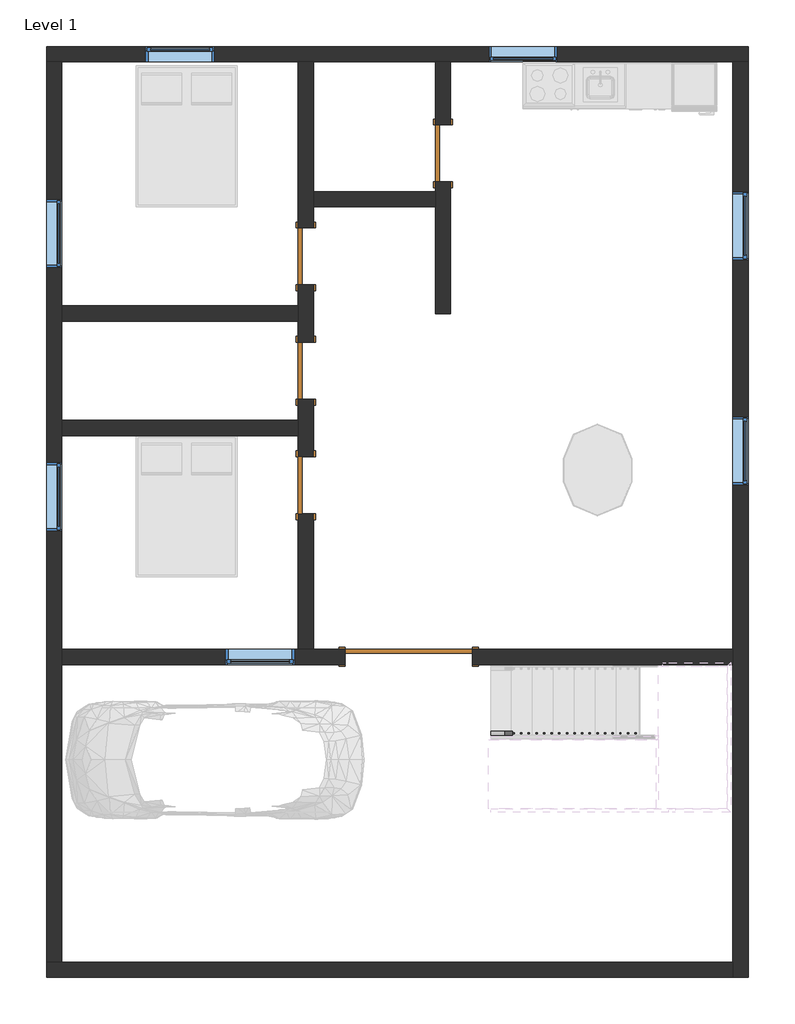
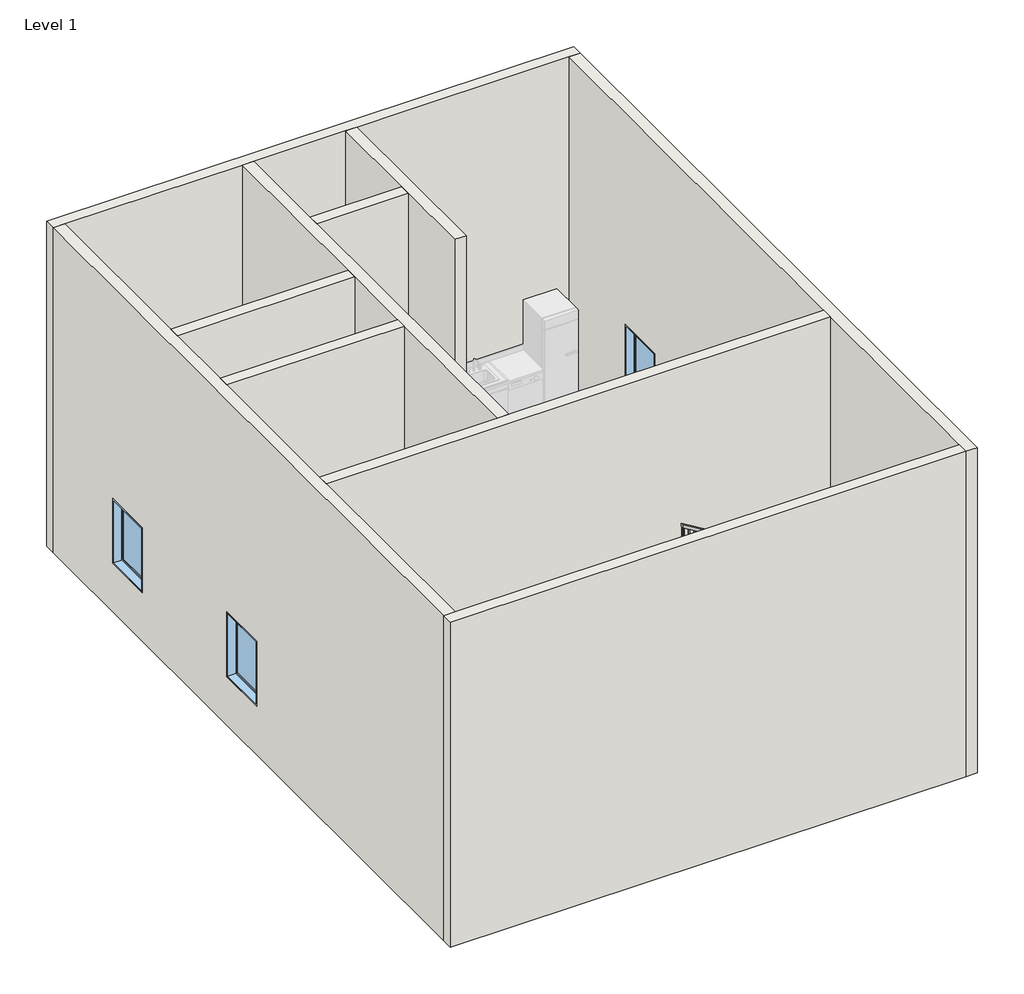
# One storey, part 1 of 2: 10 walls, 7 windows, 5 doors, 1 railing.
"""IFC4 building model written with IfcOpenShell, lengths in millimetres."""

from ifc_helpers import new_model, si_unit, frame, origin, origin_with_axes, place, context, project, spatial, polyline, outline, extrude, faceted_brep, transform, mapped, element, save
from components import m_door_double_flush_panel_double_acting_1700_x_2000mm_ee2ba557, door_53b1b562, door_fadea3f2, window_e2841890, window_9a779fa2

model = new_model("IFC4")

# Units and contexts
model_context = context("Model", 3, world=origin())
ifc_project = project(units=[si_unit("LENGTHUNIT", "METRE", prefix="MILLI")], contexts=[model_context])

# Site, building, storey
site = spatial("IfcSite", under=ifc_project)
building = spatial("IfcBuilding", under=site)
storey = spatial("IfcBuildingStorey", under=building, Name="Level 1", Elevation=0.0)

# Doors
placement = place(None, origin())
m_door_double_flush_panel_double_acting_1700_x_2000mm_shape = m_door_double_flush_panel_double_acting_1700_x_2000mm_ee2ba557(model_context)
element("IfcDoor", 1, ObjectType="M_Door-Double-Flush_Panel-Double-Acting : 1700 x 2000mm", at=placement, inside=storey, context=model_context, shape_type="MappedRepresentation", body=[
    mapped(m_door_double_flush_panel_double_acting_1700_x_2000mm_shape, transform((-5017.6851125, 2283.4979873, 0.0), x_axis=(1.0, 0.0, 0.0), y_axis=(0.0, 1.0, 0.0), z_axis=(0.0, 0.0, 1.0))),
])
door_shape = door_53b1b562(model_context)
element("IfcDoor", 2, ObjectType="Single-Flush : 30\" x 80\"", at=placement, inside=storey, context=model_context, shape_type="MappedRepresentation", body=[
    mapped(door_shape, transform((-4560.4851125, 8989.0979873, 0.0), x_axis=(0.0, -1.0, 0.0), y_axis=(1.0, 0.0, 0.0), z_axis=(0.0, 0.0, 1.0))),
])
element("IfcDoor", 3, ObjectType="Single-Flush : 30\" x 80\"", at=placement, inside=storey, context=model_context, shape_type="MappedRepresentation", body=[
    mapped(door_shape, transform((-6389.2851125, 7617.4979873, 0.0), x_axis=(0.0, -1.0, 0.0), y_axis=(1.0, 0.0, 0.0), z_axis=(0.0, 0.0, 1.0))),
])
door_2_shape = door_fadea3f2(model_context)
element("IfcDoor", 4, ObjectType="Single-Flush : 30\" x 80\"", at=placement, inside=storey, context=model_context, shape_type="MappedRepresentation", body=[
    mapped(door_2_shape, transform((-6389.2851125, 6093.4979873, 0.0), x_axis=(0.0, 1.0, 0.0), y_axis=(-1.0, 0.0, 0.0), z_axis=(0.0, 0.0, 1.0))),
])
element("IfcDoor", 5, ObjectType="Single-Flush : 30\" x 80\"", at=placement, inside=storey, context=model_context, shape_type="MappedRepresentation", body=[
    mapped(door_2_shape, transform((-6389.2851125, 4569.4979873, 0.0), x_axis=(0.0, 1.0, 0.0), y_axis=(-1.0, 0.0, 0.0), z_axis=(0.0, 0.0, 1.0))),
])

# Railing
element("IfcRailing", 6, ObjectType="Handrail - Rectangular", at=placement, inside=storey, context=model_context, shape_type="SolidModel", body=[
    faceted_brep([(-3925.4851125, 1292.9395264, 1083.7333333), (-3925.4851125, 1292.9395264, 1024.3318731), (-3925.4851125, 1242.1395264, 1024.3318731), (-3925.4851125, 1242.1395264, 1083.7333333), (-1766.4851125, 1292.9395264, 2392.2181818), (-1715.6851125, 1292.9395264, 2363.6046004), (-1715.6851125, 1242.1395264, 2363.6046004), (-1766.4851125, 1242.1395264, 2392.2181818), (-1766.4851125, 1292.9395264, 2438.4), (-1715.6851125, 1292.9395264, 2387.6), (-1715.6851125, 1242.1395264, 2387.6), (-1766.4851125, 1242.1395264, 2438.4), (-1639.4851125, 1292.9395264, 2438.4), (-1639.4851125, 1292.9395264, 2387.6), (-1690.2851125, 1242.1395264, 2387.6), (-1690.2851125, 1242.1395264, 2438.4), (-1639.4851125, 1165.9395264, 2438.4), (-1639.4851125, 1165.9395264, 2387.6), (-1690.2851125, 1165.9395264, 2387.6), (-1690.2851125, 1165.9395264, 2438.4), (-1639.4851125, 1153.7428815, 2438.4), (-1690.2851125, 1153.7428815, 2438.4), (-1690.2851125, 1153.7428815, 2387.6), (-1639.4851125, 1153.7428815, 2387.6)], [[[0, 1, 2, 3]], [[1, 0, 4, 5]], [[2, 1, 5, 6]], [[3, 2, 6, 7]], [[0, 3, 7, 4]], [[5, 4, 8, 9]], [[6, 5, 9, 10]], [[7, 6, 10, 11]], [[4, 7, 11, 8]], [[9, 8, 12, 13]], [[10, 9, 13, 14]], [[11, 10, 14, 15]], [[8, 11, 15, 12]], [[13, 12, 16, 17]], [[14, 13, 17, 18]], [[15, 14, 18, 19]], [[12, 15, 19, 16]], [[20, 21, 22, 23]], [[17, 16, 20, 23]], [[18, 17, 23, 22]], [[19, 18, 22, 21]], [[16, 19, 21, 20]]]),
    faceted_brep([(-1639.4851125, 1179.1428815, 2438.4), (-1639.4851125, 1128.3428815, 2387.6), (-1690.2851125, 1128.3428815, 2387.6), (-1690.2851125, 1179.1428815, 2438.4), (-1639.4851125, 1179.1428815, 2576.9454545), (-1690.2851125, 1179.1428815, 2548.3318731), (-1690.2851125, 1128.3428815, 2548.3318731), (-1639.4851125, 1128.3428815, 2576.9454545)], [[[0, 1, 2, 3]], [[4, 5, 6, 7]], [[1, 0, 4, 7]], [[2, 1, 7, 6]], [[3, 2, 6, 5]], [[0, 3, 5, 4]]]),
    faceted_brep([(-1639.4851125, 1128.3428815, 2576.9454545), (-1690.2851125, 1128.3428815, 2548.3318731), (-1690.2851125, 1179.1428815, 2548.3318731), (-1639.4851125, 1179.1428815, 2576.9454545), (-3925.4851125, 1128.3428815, 3962.4), (-3925.4851125, 1179.1428815, 3962.4), (-3925.4851125, 1179.1428815, 3902.9985397), (-3925.4851125, 1128.3428815, 3902.9985397)], [[[0, 1, 2, 3]], [[4, 5, 6, 7]], [[1, 0, 4, 7]], [[2, 1, 7, 6]], [[3, 2, 6, 5]], [[0, 3, 5, 4]]]),
    extrude(outline(polyline([(3881.8318731, -3890.5601125), (3893.3773276, -3909.6101125), (2878.6666667, -3909.6101125), (2878.6666667, -3890.5601125), (3881.8318731, -3890.5601125)])), frame((0.0, 1144.2178815, 0.0), z_axis=(0.0, 1.0, 0.0), x_axis=(0.0, 0.0, 1.0)), (0.0, 0.0, 1.0), 19.05),
    extrude(outline(polyline([(3820.2561155, -3788.9601125), (3831.80157, -3808.0101125), (2878.6666667, -3808.0101125), (2878.6666667, -3788.9601125), (3820.2561155, -3788.9601125)])), frame((0.0, 1144.2178815, 0.0), z_axis=(0.0, 1.0, 0.0), x_axis=(0.0, 0.0, 1.0)), (0.0, 0.0, 1.0), 19.05),
    extrude(outline(polyline([(3758.6803579, -3687.3601125), (3770.2258125, -3706.4101125), (2878.6666667, -3706.4101125), (2878.6666667, -3687.3601125), (3758.6803579, -3687.3601125)])), frame((0.0, 1144.2178815, 0.0), z_axis=(0.0, 1.0, 0.0), x_axis=(0.0, 0.0, 1.0)), (0.0, 0.0, 1.0), 19.05),
    extrude(outline(polyline([(3697.1046004, -3585.7601125), (3708.6500549, -3604.8101125), (2709.3333333, -3604.8101125), (2709.3333333, -3585.7601125), (3697.1046004, -3585.7601125)])), frame((0.0, 1144.2178815, 0.0), z_axis=(0.0, 1.0, 0.0), x_axis=(0.0, 0.0, 1.0)), (0.0, 0.0, 1.0), 19.05),
    extrude(outline(polyline([(3635.5288428, -3484.1601125), (3647.0742973, -3503.2101125), (2709.3333333, -3503.2101125), (2709.3333333, -3484.1601125), (3635.5288428, -3484.1601125)])), frame((0.0, 1144.2178815, 0.0), z_axis=(0.0, 1.0, 0.0), x_axis=(0.0, 0.0, 1.0)), (0.0, 0.0, 1.0), 19.05),
    extrude(outline(polyline([(3573.9530852, -3382.5601125), (3585.4985397, -3401.6101125), (2709.3333333, -3401.6101125), (2709.3333333, -3382.5601125), (3573.9530852, -3382.5601125)])), frame((0.0, 1144.2178815, 0.0), z_axis=(0.0, 1.0, 0.0), x_axis=(0.0, 0.0, 1.0)), (0.0, 0.0, 1.0), 19.05),
    extrude(outline(polyline([(3512.3773276, -3280.9601125), (3523.9227822, -3300.0101125), (2540.0, -3300.0101125), (2540.0, -3280.9601125), (3512.3773276, -3280.9601125)])), frame((0.0, 1144.2178815, 0.0), z_axis=(0.0, 1.0, 0.0), x_axis=(0.0, 0.0, 1.0)), (0.0, 0.0, 1.0), 19.05),
    extrude(outline(polyline([(3450.80157, -3179.3601125), (3462.3470246, -3198.4101125), (2540.0, -3198.4101125), (2540.0, -3179.3601125), (3450.80157, -3179.3601125)])), frame((0.0, 1144.2178815, 0.0), z_axis=(0.0, 1.0, 0.0), x_axis=(0.0, 0.0, 1.0)), (0.0, 0.0, 1.0), 19.05),
    extrude(outline(polyline([(3389.2258125, -3077.7601125), (3400.771267, -3096.8101125), (2540.0, -3096.8101125), (2540.0, -3077.7601125), (3389.2258125, -3077.7601125)])), frame((0.0, 1144.2178815, 0.0), z_axis=(0.0, 1.0, 0.0), x_axis=(0.0, 0.0, 1.0)), (0.0, 0.0, 1.0), 19.05),
    extrude(outline(polyline([(3327.6500549, -2976.1601125), (3339.1955094, -2995.2101125), (2370.6666667, -2995.2101125), (2370.6666667, -2976.1601125), (3327.6500549, -2976.1601125)])), frame((0.0, 1144.2178815, 0.0), z_axis=(0.0, 1.0, 0.0), x_axis=(0.0, 0.0, 1.0)), (0.0, 0.0, 1.0), 19.05),
    extrude(outline(polyline([(3266.0742973, -2874.5601125), (3277.6197519, -2893.6101125), (2370.6666667, -2893.6101125), (2370.6666667, -2874.5601125), (3266.0742973, -2874.5601125)])), frame((0.0, 1144.2178815, 0.0), z_axis=(0.0, 1.0, 0.0), x_axis=(0.0, 0.0, 1.0)), (0.0, 0.0, 1.0), 19.05),
    extrude(outline(polyline([(3204.4985397, -2772.9601125), (3216.0439943, -2792.0101125), (2201.3333333, -2792.0101125), (2201.3333333, -2772.9601125), (3204.4985397, -2772.9601125)])), frame((0.0, 1144.2178815, 0.0), z_axis=(0.0, 1.0, 0.0), x_axis=(0.0, 0.0, 1.0)), (0.0, 0.0, 1.0), 19.05),
    extrude(outline(polyline([(3142.9227822, -2671.3601125), (3154.4682367, -2690.4101125), (2201.3333333, -2690.4101125), (2201.3333333, -2671.3601125), (3142.9227822, -2671.3601125)])), frame((0.0, 1144.2178815, 0.0), z_axis=(0.0, 1.0, 0.0), x_axis=(0.0, 0.0, 1.0)), (0.0, 0.0, 1.0), 19.05),
    extrude(outline(polyline([(3081.3470246, -2569.7601125), (3092.8924791, -2588.8101125), (2201.3333333, -2588.8101125), (2201.3333333, -2569.7601125), (3081.3470246, -2569.7601125)])), frame((0.0, 1144.2178815, 0.0), z_axis=(0.0, 1.0, 0.0), x_axis=(0.0, 0.0, 1.0)), (0.0, 0.0, 1.0), 19.05),
    extrude(outline(polyline([(3019.771267, -2468.1601125), (3031.3167216, -2487.2101125), (2032.0, -2487.2101125), (2032.0, -2468.1601125), (3019.771267, -2468.1601125)])), frame((0.0, 1144.2178815, 0.0), z_axis=(0.0, 1.0, 0.0), x_axis=(0.0, 0.0, 1.0)), (0.0, 0.0, 1.0), 19.05),
    extrude(outline(polyline([(2958.1955094, -2366.5601125), (2969.740964, -2385.6101125), (2032.0, -2385.6101125), (2032.0, -2366.5601125), (2958.1955094, -2366.5601125)])), frame((0.0, 1144.2178815, 0.0), z_axis=(0.0, 1.0, 0.0), x_axis=(0.0, 0.0, 1.0)), (0.0, 0.0, 1.0), 19.05),
    extrude(outline(polyline([(2896.6197519, -2264.9601125), (2908.1652064, -2284.0101125), (2032.0, -2284.0101125), (2032.0, -2264.9601125), (2896.6197519, -2264.9601125)])), frame((0.0, 1144.2178815, 0.0), z_axis=(0.0, 1.0, 0.0), x_axis=(0.0, 0.0, 1.0)), (0.0, 0.0, 1.0), 19.05),
    extrude(outline(polyline([(2835.0439943, -2163.3601125), (2846.5894488, -2182.4101125), (1862.6666667, -2182.4101125), (1862.6666667, -2163.3601125), (2835.0439943, -2163.3601125)])), frame((0.0, 1144.2178815, 0.0), z_axis=(0.0, 1.0, 0.0), x_axis=(0.0, 0.0, 1.0)), (0.0, 0.0, 1.0), 19.05),
    extrude(outline(polyline([(2773.4682367, -2061.7601125), (2785.0136913, -2080.8101125), (1862.6666667, -2080.8101125), (1862.6666667, -2061.7601125), (2773.4682367, -2061.7601125)])), frame((0.0, 1144.2178815, 0.0), z_axis=(0.0, 1.0, 0.0), x_axis=(0.0, 0.0, 1.0)), (0.0, 0.0, 1.0), 19.05),
    extrude(outline(polyline([(2711.8924791, -1960.1601125), (2723.4379337, -1979.2101125), (1862.6666667, -1979.2101125), (1862.6666667, -1960.1601125), (2711.8924791, -1960.1601125)])), frame((0.0, 1144.2178815, 0.0), z_axis=(0.0, 1.0, 0.0), x_axis=(0.0, 0.0, 1.0)), (0.0, 0.0, 1.0), 19.05),
    extrude(outline(polyline([(2650.3167216, -1858.5601125), (2661.8621761, -1877.6101125), (1693.3333333, -1877.6101125), (1693.3333333, -1858.5601125), (2650.3167216, -1858.5601125)])), frame((0.0, 1144.2178815, 0.0), z_axis=(0.0, 1.0, 0.0), x_axis=(0.0, 0.0, 1.0)), (0.0, 0.0, 1.0), 19.05),
    extrude(outline(polyline([(2588.740964, -1756.9601125), (2600.2864185, -1776.0101125), (1693.3333333, -1776.0101125), (1693.3333333, -1756.9601125), (2588.740964, -1756.9601125)])), frame((0.0, 1144.2178815, 0.0), z_axis=(0.0, 1.0, 0.0), x_axis=(0.0, 0.0, 1.0)), (0.0, 0.0, 1.0), 19.05),
    extrude(outline(polyline([(-1674.4101125, 1175.4645264), (-1655.3601125, 1175.4645264), (-1655.3601125, 1156.4145264), (-1674.4101125, 1156.4145264), (-1674.4101125, 1175.4645264)])), frame((0.0, 0.0, 1524.0), z_axis=(0.0, 0.0, 1.0), x_axis=(1.0, 0.0, 0.0)), (0.0, 0.0, 1.0), 863.6),
    extrude(outline(polyline([(2323.1955094, -1782.3601125), (2311.6500549, -1801.4101125), (1354.6666667, -1801.4101125), (1354.6666667, -1782.3601125), (2323.1955094, -1782.3601125)])), frame((0.0, 1258.0145264, 0.0), z_axis=(0.0, 1.0, 0.0), x_axis=(0.0, 0.0, 1.0)), (0.0, 0.0, 1.0), 19.05),
    extrude(outline(polyline([(2261.6197519, -1883.9601125), (2250.0742973, -1903.0101125), (1354.6666667, -1903.0101125), (1354.6666667, -1883.9601125), (2261.6197519, -1883.9601125)])), frame((0.0, 1258.0145264, 0.0), z_axis=(0.0, 1.0, 0.0), x_axis=(0.0, 0.0, 1.0)), (0.0, 0.0, 1.0), 19.05),
    extrude(outline(polyline([(2200.0439943, -1985.5601125), (2188.4985397, -2004.6101125), (1185.3333333, -2004.6101125), (1185.3333333, -1985.5601125), (2200.0439943, -1985.5601125)])), frame((0.0, 1258.0145264, 0.0), z_axis=(0.0, 1.0, 0.0), x_axis=(0.0, 0.0, 1.0)), (0.0, 0.0, 1.0), 19.05),
    extrude(outline(polyline([(2138.4682367, -2087.1601125), (2126.9227822, -2106.2101125), (1185.3333333, -2106.2101125), (1185.3333333, -2087.1601125), (2138.4682367, -2087.1601125)])), frame((0.0, 1258.0145264, 0.0), z_axis=(0.0, 1.0, 0.0), x_axis=(0.0, 0.0, 1.0)), (0.0, 0.0, 1.0), 19.05),
    extrude(outline(polyline([(2076.8924791, -2188.7601125), (2065.3470246, -2207.8101125), (1185.3333333, -2207.8101125), (1185.3333333, -2188.7601125), (2076.8924791, -2188.7601125)])), frame((0.0, 1258.0145264, 0.0), z_axis=(0.0, 1.0, 0.0), x_axis=(0.0, 0.0, 1.0)), (0.0, 0.0, 1.0), 19.05),
    extrude(outline(polyline([(2015.3167216, -2290.3601125), (2003.771267, -2309.4101125), (1016.0, -2309.4101125), (1016.0, -2290.3601125), (2015.3167216, -2290.3601125)])), frame((0.0, 1258.0145264, 0.0), z_axis=(0.0, 1.0, 0.0), x_axis=(0.0, 0.0, 1.0)), (0.0, 0.0, 1.0), 19.05),
    extrude(outline(polyline([(1953.740964, -2391.9601125), (1942.1955094, -2411.0101125), (1016.0, -2411.0101125), (1016.0, -2391.9601125), (1953.740964, -2391.9601125)])), frame((0.0, 1258.0145264, 0.0), z_axis=(0.0, 1.0, 0.0), x_axis=(0.0, 0.0, 1.0)), (0.0, 0.0, 1.0), 19.05),
    extrude(outline(polyline([(1892.1652064, -2493.5601125), (1880.6197519, -2512.6101125), (1016.0, -2512.6101125), (1016.0, -2493.5601125), (1892.1652064, -2493.5601125)])), frame((0.0, 1258.0145264, 0.0), z_axis=(0.0, 1.0, 0.0), x_axis=(0.0, 0.0, 1.0)), (0.0, 0.0, 1.0), 19.05),
    extrude(outline(polyline([(1830.5894488, -2595.1601125), (1819.0439943, -2614.2101125), (846.6666667, -2614.2101125), (846.6666667, -2595.1601125), (1830.5894488, -2595.1601125)])), frame((0.0, 1258.0145264, 0.0), z_axis=(0.0, 1.0, 0.0), x_axis=(0.0, 0.0, 1.0)), (0.0, 0.0, 1.0), 19.05),
    extrude(outline(polyline([(1769.0136913, -2696.7601125), (1757.4682367, -2715.8101125), (846.6666667, -2715.8101125), (846.6666667, -2696.7601125), (1769.0136913, -2696.7601125)])), frame((0.0, 1258.0145264, 0.0), z_axis=(0.0, 1.0, 0.0), x_axis=(0.0, 0.0, 1.0)), (0.0, 0.0, 1.0), 19.05),
    extrude(outline(polyline([(1707.4379337, -2798.3601125), (1695.8924791, -2817.4101125), (846.6666667, -2817.4101125), (846.6666667, -2798.3601125), (1707.4379337, -2798.3601125)])), frame((0.0, 1258.0145264, 0.0), z_axis=(0.0, 1.0, 0.0), x_axis=(0.0, 0.0, 1.0)), (0.0, 0.0, 1.0), 19.05),
    extrude(outline(polyline([(1645.8621761, -2899.9601125), (1634.3167216, -2919.0101125), (677.3333333, -2919.0101125), (677.3333333, -2899.9601125), (1645.8621761, -2899.9601125)])), frame((0.0, 1258.0145264, 0.0), z_axis=(0.0, 1.0, 0.0), x_axis=(0.0, 0.0, 1.0)), (0.0, 0.0, 1.0), 19.05),
    extrude(outline(polyline([(1584.2864185, -3001.5601125), (1572.740964, -3020.6101125), (677.3333333, -3020.6101125), (677.3333333, -3001.5601125), (1584.2864185, -3001.5601125)])), frame((0.0, 1258.0145264, 0.0), z_axis=(0.0, 1.0, 0.0), x_axis=(0.0, 0.0, 1.0)), (0.0, 0.0, 1.0), 19.05),
    extrude(outline(polyline([(1522.710661, -3103.1601125), (1511.1652064, -3122.2101125), (508.0, -3122.2101125), (508.0, -3103.1601125), (1522.710661, -3103.1601125)])), frame((0.0, 1258.0145264, 0.0), z_axis=(0.0, 1.0, 0.0), x_axis=(0.0, 0.0, 1.0)), (0.0, 0.0, 1.0), 19.05),
    extrude(outline(polyline([(1461.1349034, -3204.7601125), (1449.5894488, -3223.8101125), (508.0, -3223.8101125), (508.0, -3204.7601125), (1461.1349034, -3204.7601125)])), frame((0.0, 1258.0145264, 0.0), z_axis=(0.0, 1.0, 0.0), x_axis=(0.0, 0.0, 1.0)), (0.0, 0.0, 1.0), 19.05),
    extrude(outline(polyline([(1399.5591458, -3306.3601125), (1388.0136913, -3325.4101125), (508.0, -3325.4101125), (508.0, -3306.3601125), (1399.5591458, -3306.3601125)])), frame((0.0, 1258.0145264, 0.0), z_axis=(0.0, 1.0, 0.0), x_axis=(0.0, 0.0, 1.0)), (0.0, 0.0, 1.0), 19.05),
    extrude(outline(polyline([(1337.9833882, -3407.9601125), (1326.4379337, -3427.0101125), (338.6666667, -3427.0101125), (338.6666667, -3407.9601125), (1337.9833882, -3407.9601125)])), frame((0.0, 1258.0145264, 0.0), z_axis=(0.0, 1.0, 0.0), x_axis=(0.0, 0.0, 1.0)), (0.0, 0.0, 1.0), 19.05),
    extrude(outline(polyline([(1276.4076307, -3509.5601125), (1264.8621761, -3528.6101125), (338.6666667, -3528.6101125), (338.6666667, -3509.5601125), (1276.4076307, -3509.5601125)])), frame((0.0, 1258.0145264, 0.0), z_axis=(0.0, 1.0, 0.0), x_axis=(0.0, 0.0, 1.0)), (0.0, 0.0, 1.0), 19.05),
    extrude(outline(polyline([(1214.8318731, -3611.1601125), (1203.2864185, -3630.2101125), (338.6666667, -3630.2101125), (338.6666667, -3611.1601125), (1214.8318731, -3611.1601125)])), frame((0.0, 1258.0145264, 0.0), z_axis=(0.0, 1.0, 0.0), x_axis=(0.0, 0.0, 1.0)), (0.0, 0.0, 1.0), 19.05),
    extrude(outline(polyline([(1153.2561155, -3712.7601125), (1141.710661, -3731.8101125), (169.3333333, -3731.8101125), (169.3333333, -3712.7601125), (1153.2561155, -3712.7601125)])), frame((0.0, 1258.0145264, 0.0), z_axis=(0.0, 1.0, 0.0), x_axis=(0.0, 0.0, 1.0)), (0.0, 0.0, 1.0), 19.05),
    extrude(outline(polyline([(1091.6803579, -3814.3601125), (1080.1349034, -3833.4101125), (169.3333333, -3833.4101125), (169.3333333, -3814.3601125), (1091.6803579, -3814.3601125)])), frame((0.0, 1258.0145264, 0.0), z_axis=(0.0, 1.0, 0.0), x_axis=(0.0, 0.0, 1.0)), (0.0, 0.0, 1.0), 19.05),
    extrude(outline(polyline([(-1655.3601125, 1163.2678815), (-1655.3601125, 1144.2178815), (-1674.4101125, 1144.2178815), (-1674.4101125, 1163.2678815), (-1655.3601125, 1163.2678815)])), frame((0.0, 0.0, 1524.0), z_axis=(0.0, 0.0, 1.0), x_axis=(1.0, 0.0, 0.0)), (0.0, 0.0, 1.0), 863.6),
    extrude(outline(polyline([(-1674.4101125, 1258.0145264), (-1674.4101125, 1277.0645264), (-1655.3601125, 1277.0645264), (-1655.3601125, 1258.0145264), (-1674.4101125, 1258.0145264)])), frame((0.0, 0.0, 1524.0), z_axis=(0.0, 0.0, 1.0), x_axis=(1.0, 0.0, 0.0)), (0.0, 0.0, 1.0), 863.6),
    extrude(outline(polyline([(-1699.8101125, 1258.0145264), (-1699.8101125, 1277.0645264), (-1680.7601125, 1277.0645264), (-1680.7601125, 1258.0145264), (-1699.8101125, 1258.0145264)])), frame((0.0, 0.0, 1524.0), z_axis=(0.0, 0.0, 1.0), x_axis=(1.0, 0.0, 0.0)), (0.0, 0.0, 1.0), 863.6),
    extrude(outline(polyline([(3891.4530852, -3906.4351125), (3902.9985397, -3925.4851125), (2878.6666667, -3925.4851125), (2878.6666667, -3906.4351125), (3891.4530852, -3906.4351125)])), frame((0.0, 1144.2178815, 0.0), z_axis=(0.0, 1.0, 0.0), x_axis=(0.0, 0.0, 1.0)), (0.0, 0.0, 1.0), 19.05),
    extrude(outline(polyline([(1035.8773276, -3906.4351125), (1024.3318731, -3925.4851125), (169.3333333, -3925.4851125), (169.3333333, -3906.4351125), (1035.8773276, -3906.4351125)])), frame((0.0, 1258.0145264, 0.0), z_axis=(0.0, 1.0, 0.0), x_axis=(0.0, 0.0, 1.0)), (0.0, 0.0, 1.0), 19.05),
])

# Walls
element("IfcWall", 7, ObjectType="Generic - 8\"", at=placement, inside=storey, context=model_context, shape_type="Brep", body=[
    faceted_brep([(-9843.6851125, 10208.2979873, 0.0), (-9640.4851125, 10208.2979873, 0.0), (-6490.8851125, 10208.2979873, 0.0), (-6287.6851125, 10208.2979873, 0.0), (-4662.0851125, 10208.2979873, 0.0), (-4458.8851125, 10208.2979873, 0.0), (-699.6851125, 10208.2979873, 0.0), (-496.4851125, 10208.2979873, 0.0), (-496.4851125, 10208.2979873, 6096.0), (-699.6851125, 10208.2979873, 6096.0), (-4458.8851125, 10208.2979873, 6096.0), (-4662.0851125, 10208.2979873, 6096.0), (-6287.6851125, 10208.2979873, 6096.0), (-6490.8851125, 10208.2979873, 6096.0), (-9640.4851125, 10208.2979873, 6096.0), (-9843.6851125, 10208.2979873, 6096.0), (-7608.4851125, 10208.2979873, 2133.6), (-7608.4851125, 10208.2979873, 914.4), (-8522.8851125, 10208.2979873, 914.4), (-8522.8851125, 10208.2979873, 2133.6), (-3950.8851125, 10208.2979873, 2133.6), (-3036.4851125, 10208.2979873, 2133.6), (-3036.4851125, 10208.2979873, 304.8), (-3950.8851125, 10208.2979873, 304.8), (-9843.6851125, 10411.4979873, 0.0), (-9843.6851125, 10411.4979873, 6096.0), (-496.4851125, 10411.4979873, 6096.0), (-496.4851125, 10411.4979873, 0.0), (-7608.4851125, 10411.4979873, 2133.6), (-8522.8851125, 10411.4979873, 2133.6), (-8522.8851125, 10411.4979873, 914.4), (-7608.4851125, 10411.4979873, 914.4), (-3950.8851125, 10411.4979873, 2133.6), (-3950.8851125, 10411.4979873, 304.8), (-3036.4851125, 10411.4979873, 304.8), (-3036.4851125, 10411.4979873, 2133.6)], [[[0, 1, 2, 3, 4, 5, 6, 7, 8, 9, 10, 11, 12, 13, 14, 15], [16, 17, 18, 19], [20, 21, 22, 23]], [[24, 25, 26, 27], [28, 29, 30, 31], [32, 33, 34, 35]], [[7, 6, 5, 4, 3, 2, 1, 0, 24, 27]], [[15, 14, 13, 12, 11, 10, 9, 8, 26, 25]], [[8, 7, 27, 26]], [[0, 15, 25, 24]], [[17, 16, 28, 31]], [[18, 17, 31, 30]], [[19, 18, 30, 29]], [[16, 19, 29, 28]], [[33, 32, 20, 23]], [[34, 33, 23, 22]], [[35, 34, 22, 21]], [[32, 35, 21, 20]]]),
])
element("IfcWall", 8, ObjectType="Generic - 8\"", at=placement, inside=storey, context=model_context, shape_type="Brep", body=[
    faceted_brep([(-699.6851125, 10208.2979873, 0.0), (-699.6851125, 2385.0979873, 0.0), (-699.6851125, 2181.8979873, 0.0), (-699.6851125, -1780.5020127, 0.0), (-699.6851125, -1983.7020127, 0.0), (-699.6851125, -1983.7020127, 6096.0), (-699.6851125, -1780.5020127, 6096.0), (-699.6851125, 2181.8979873, 6096.0), (-699.6851125, 2385.0979873, 6096.0), (-699.6851125, 10208.2979873, 6096.0), (-699.6851125, 4569.4979873, 2133.6), (-699.6851125, 4569.4979873, 304.8), (-699.6851125, 5483.8979873, 304.8), (-699.6851125, 5483.8979873, 2133.6), (-699.6851125, 7566.6979873, 2133.6), (-699.6851125, 7566.6979873, 304.8), (-699.6851125, 8481.0979873, 304.8), (-699.6851125, 8481.0979873, 2133.6), (-496.4851125, 10208.2979873, 0.0), (-496.4851125, 10208.2979873, 6096.0), (-496.4851125, -1983.7020127, 6096.0), (-496.4851125, -1983.7020127, 0.0), (-496.4851125, 4569.4979873, 2133.6), (-496.4851125, 5483.8979873, 2133.6), (-496.4851125, 5483.8979873, 304.8), (-496.4851125, 4569.4979873, 304.8), (-496.4851125, 7566.6979873, 2133.6), (-496.4851125, 8481.0979873, 2133.6), (-496.4851125, 8481.0979873, 304.8), (-496.4851125, 7566.6979873, 304.8)], [[[0, 1, 2, 3, 4, 5, 6, 7, 8, 9], [10, 11, 12, 13], [14, 15, 16, 17]], [[18, 19, 20, 21], [22, 23, 24, 25], [26, 27, 28, 29]], [[4, 3, 2, 1, 0, 18, 21]], [[9, 8, 7, 6, 5, 20, 19]], [[0, 9, 19, 18]], [[5, 4, 21, 20]], [[11, 10, 22, 25]], [[12, 11, 25, 24]], [[13, 12, 24, 23]], [[10, 13, 23, 22]], [[15, 14, 26, 29]], [[16, 15, 29, 28]], [[17, 16, 28, 27]], [[14, 17, 27, 26]]]),
])
element("IfcWall", 9, ObjectType="Generic - 8\"", at=placement, inside=storey, context=model_context, shape_type="Brep", body=[
    faceted_brep([(-699.6851125, -1780.5020127, 0.0), (-9640.4851125, -1780.5020127, 0.0), (-9843.6851125, -1780.5020127, 0.0), (-9843.6851125, -1780.5020127, 6096.0), (-9640.4851125, -1780.5020127, 6096.0), (-699.6851125, -1780.5020127, 6096.0), (-699.6851125, -1983.7020127, 0.0), (-699.6851125, -1983.7020127, 6096.0), (-9843.6851125, -1983.7020127, 6096.0), (-9843.6851125, -1983.7020127, 0.0)], [[[0, 1, 2, 3, 4, 5]], [[6, 7, 8, 9]], [[2, 1, 0, 6, 9]], [[5, 4, 3, 8, 7]], [[0, 5, 7, 6]], [[3, 2, 9, 8]]]),
])
element("IfcWall", 10, ObjectType="Generic - 8\"", at=placement, inside=storey, context=model_context, shape_type="Brep", body=[
    faceted_brep([(-9640.4851125, -1780.5020127, 0.0), (-9640.4851125, 2181.8979873, 0.0), (-9640.4851125, 2385.0979873, 0.0), (-9640.4851125, 5229.8979873, 0.0), (-9640.4851125, 5433.0979873, 0.0), (-9640.4851125, 6753.8979873, 0.0), (-9640.4851125, 6957.0979873, 0.0), (-9640.4851125, 10208.2979873, 0.0), (-9640.4851125, 10208.2979873, 6096.0), (-9640.4851125, 6957.0979873, 6096.0), (-9640.4851125, 6753.8979873, 6096.0), (-9640.4851125, 5433.0979873, 6096.0), (-9640.4851125, 5229.8979873, 6096.0), (-9640.4851125, 2385.0979873, 6096.0), (-9640.4851125, 2181.8979873, 6096.0), (-9640.4851125, -1780.5020127, 6096.0), (-9640.4851125, 7465.0979873, 2133.6), (-9640.4851125, 8379.4979873, 2133.6), (-9640.4851125, 8379.4979873, 914.4), (-9640.4851125, 7465.0979873, 914.4), (-9640.4851125, 3959.8979873, 2133.6), (-9640.4851125, 4874.2979873, 2133.6), (-9640.4851125, 4874.2979873, 914.4), (-9640.4851125, 3959.8979873, 914.4), (-9843.6851125, -1780.5020127, 0.0), (-9843.6851125, -1780.5020127, 6096.0), (-9843.6851125, 10208.2979873, 6096.0), (-9843.6851125, 10208.2979873, 0.0), (-9843.6851125, 7465.0979873, 2133.6), (-9843.6851125, 7465.0979873, 914.4), (-9843.6851125, 8379.4979873, 914.4), (-9843.6851125, 8379.4979873, 2133.6), (-9843.6851125, 3959.8979873, 2133.6), (-9843.6851125, 3959.8979873, 914.4), (-9843.6851125, 4874.2979873, 914.4), (-9843.6851125, 4874.2979873, 2133.6)], [[[0, 1, 2, 3, 4, 5, 6, 7, 8, 9, 10, 11, 12, 13, 14, 15], [16, 17, 18, 19], [20, 21, 22, 23]], [[24, 25, 26, 27], [28, 29, 30, 31], [32, 33, 34, 35]], [[7, 6, 5, 4, 3, 2, 1, 0, 24, 27]], [[15, 14, 13, 12, 11, 10, 9, 8, 26, 25]], [[8, 7, 27, 26]], [[0, 15, 25, 24]], [[29, 28, 16, 19]], [[30, 29, 19, 18]], [[31, 30, 18, 17]], [[28, 31, 17, 16]], [[33, 32, 20, 23]], [[34, 33, 23, 22]], [[35, 34, 22, 21]], [[32, 35, 21, 20]]]),
])
element("IfcWall", 11, ObjectType="Generic - 8\"", at=placement, inside=storey, context=model_context, shape_type="Brep", body=[
    faceted_brep([(-6490.8851125, 7236.4979873, 2032.0), (-6490.8851125, 7236.4979873, 0.0), (-6490.8851125, 6957.0979873, 0.0), (-6490.8851125, 6753.8979873, 0.0), (-6490.8851125, 6474.4979873, 0.0), (-6490.8851125, 6474.4979873, 2032.0), (-6490.8851125, 5712.4979873, 2032.0), (-6490.8851125, 5712.4979873, 0.0), (-6490.8851125, 5433.0979873, 0.0), (-6490.8851125, 5229.8979873, 0.0), (-6490.8851125, 4950.4979873, 0.0), (-6490.8851125, 4950.4979873, 2032.0), (-6490.8851125, 4188.4979873, 2032.0), (-6490.8851125, 4188.4979873, 0.0), (-6490.8851125, 2385.0979873, 0.0), (-6490.8851125, 2385.0979873, 6096.0), (-6490.8851125, 5229.8979873, 6096.0), (-6490.8851125, 5433.0979873, 6096.0), (-6490.8851125, 6753.8979873, 6096.0), (-6490.8851125, 6957.0979873, 6096.0), (-6490.8851125, 10208.2979873, 6096.0), (-6490.8851125, 10208.2979873, 0.0), (-6490.8851125, 7998.4979873, 0.0), (-6490.8851125, 7998.4979873, 2032.0), (-6287.6851125, 6474.4979873, 0.0), (-6287.6851125, 7236.4979873, 0.0), (-6287.6851125, 7236.4979873, 2032.0), (-6287.6851125, 7998.4979873, 2032.0), (-6287.6851125, 7998.4979873, 0.0), (-6287.6851125, 8277.8979873, 0.0), (-6287.6851125, 8481.0979873, 0.0), (-6287.6851125, 10208.2979873, 0.0), (-6287.6851125, 10208.2979873, 6096.0), (-6287.6851125, 8481.0979873, 6096.0), (-6287.6851125, 8277.8979873, 6096.0), (-6287.6851125, 2385.0979873, 6096.0), (-6287.6851125, 2385.0979873, 0.0), (-6287.6851125, 4188.4979873, 0.0), (-6287.6851125, 4188.4979873, 2032.0), (-6287.6851125, 4950.4979873, 2032.0), (-6287.6851125, 4950.4979873, 0.0), (-6287.6851125, 5712.4979873, 0.0), (-6287.6851125, 5712.4979873, 2032.0), (-6287.6851125, 6474.4979873, 2032.0)], [[[0, 1, 2, 3, 4, 5, 6, 7, 8, 9, 10, 11, 12, 13, 14, 15, 16, 17, 18, 19, 20, 21, 22, 23]], [[24, 25, 26, 27, 28, 29, 30, 31, 32, 33, 34, 35, 36, 37, 38, 39, 40, 41, 42, 43]], [[37, 36, 14, 13]], [[41, 40, 10, 9, 8, 7]], [[22, 21, 31, 30, 29, 28]], [[4, 3, 2, 1, 25, 24]], [[20, 19, 18, 17, 16, 15, 35, 34, 33, 32]], [[21, 20, 32, 31]], [[15, 14, 36, 35]], [[5, 4, 24, 43]], [[6, 5, 43, 42]], [[7, 6, 42, 41]], [[11, 10, 40, 39]], [[12, 11, 39, 38]], [[13, 12, 38, 37]], [[26, 25, 1, 0]], [[27, 26, 0, 23]], [[28, 27, 23, 22]]]),
])
element("IfcWall", 12, ObjectType="Generic - 8\"", at=placement, inside=storey, context=model_context, shape_type="SweptSolid", body=[
    extrude(outline(polyline([(-9640.4851125, 6957.0979873), (-6490.8851125, 6957.0979873), (-6490.8851125, 6753.8979873), (-9640.4851125, 6753.8979873), (-9640.4851125, 6957.0979873)])), origin_with_axes(), (0.0, 0.0, 1.0), 6096.0),
])
element("IfcWall", 13, ObjectType="Generic - 8\"", at=placement, inside=storey, context=model_context, shape_type="Brep", body=[
    faceted_brep([(-4662.0851125, 8608.0979873, 2032.0), (-4662.0851125, 8608.0979873, 0.0), (-4662.0851125, 8481.0979873, 0.0), (-4662.0851125, 8277.8979873, 0.0), (-4662.0851125, 6855.4979873, 0.0), (-4662.0851125, 6855.4979873, 6096.0), (-4662.0851125, 8277.8979873, 6096.0), (-4662.0851125, 8481.0979873, 6096.0), (-4662.0851125, 10208.2979873, 6096.0), (-4662.0851125, 10208.2979873, 0.0), (-4662.0851125, 9370.0979873, 0.0), (-4662.0851125, 9370.0979873, 2032.0), (-4458.8851125, 6855.4979873, 0.0), (-4458.8851125, 8608.0979873, 0.0), (-4458.8851125, 8608.0979873, 2032.0), (-4458.8851125, 9370.0979873, 2032.0), (-4458.8851125, 9370.0979873, 0.0), (-4458.8851125, 10208.2979873, 0.0), (-4458.8851125, 10208.2979873, 6096.0), (-4458.8851125, 6855.4979873, 6096.0)], [[[0, 1, 2, 3, 4, 5, 6, 7, 8, 9, 10, 11]], [[12, 13, 14, 15, 16, 17, 18, 19]], [[10, 9, 17, 16]], [[4, 3, 2, 1, 13, 12]], [[5, 4, 12, 19]], [[8, 7, 6, 5, 19, 18]], [[9, 8, 18, 17]], [[14, 13, 1, 0]], [[15, 14, 0, 11]], [[16, 15, 11, 10]]]),
])
element("IfcWall", 14, ObjectType="Generic - 8\"", at=placement, inside=storey, context=model_context, shape_type="SweptSolid", body=[
    extrude(outline(polyline([(-6287.6851125, 8481.0979873), (-4662.0851125, 8481.0979873), (-4662.0851125, 8277.8979873), (-6287.6851125, 8277.8979873), (-6287.6851125, 8481.0979873)])), origin_with_axes(), (0.0, 0.0, 1.0), 6096.0),
])
element("IfcWall", 15, ObjectType="Generic - 8\"", at=placement, inside=storey, context=model_context, shape_type="SweptSolid", body=[
    extrude(outline(polyline([(-6490.8851125, 5229.8979873), (-9640.4851125, 5229.8979873), (-9640.4851125, 5433.0979873), (-6490.8851125, 5433.0979873), (-6490.8851125, 5229.8979873)])), origin_with_axes(), (0.0, 0.0, 1.0), 6096.0),
])
element("IfcWall", 16, ObjectType="Generic - 8\"", at=placement, inside=storey, context=model_context, shape_type="Brep", body=[
    faceted_brep([(-699.6851125, 2181.8979873, 6096.0), (-9640.4851125, 2181.8979873, 6096.0), (-9640.4851125, 2181.8979873, 0.0), (-5867.6851125, 2181.8979873, 0.0), (-5867.6851125, 2181.8979873, 2000.0), (-4167.6851125, 2181.8979873, 2000.0), (-4167.6851125, 2181.8979873, 0.0), (-699.6851125, 2181.8979873, 0.0), (-7456.0851125, 2181.8979873, 2133.6), (-6541.6851125, 2181.8979873, 2133.6), (-6541.6851125, 2181.8979873, 914.4), (-7456.0851125, 2181.8979873, 914.4), (-9640.4851125, 2385.0979873, 6096.0), (-6490.8851125, 2385.0979873, 6096.0), (-6287.6851125, 2385.0979873, 6096.0), (-699.6851125, 2385.0979873, 6096.0), (-699.6851125, 2385.0979873, 0.0), (-4167.6851125, 2385.0979873, 0.0), (-4167.6851125, 2385.0979873, 2000.0), (-5867.6851125, 2385.0979873, 2000.0), (-5867.6851125, 2385.0979873, 0.0), (-6287.6851125, 2385.0979873, 0.0), (-6490.8851125, 2385.0979873, 0.0), (-9640.4851125, 2385.0979873, 0.0), (-7456.0851125, 2385.0979873, 2133.6), (-7456.0851125, 2385.0979873, 914.4), (-6541.6851125, 2385.0979873, 914.4), (-6541.6851125, 2385.0979873, 2133.6)], [[[0, 1, 2, 3, 4, 5, 6, 7], [8, 9, 10, 11]], [[12, 13, 14, 15, 16, 17, 18, 19, 20, 21, 22, 23], [24, 25, 26, 27]], [[2, 23, 22, 21, 20, 3]], [[16, 7, 6, 17]], [[1, 0, 15, 14, 13, 12]], [[2, 1, 12, 23]], [[0, 7, 16, 15]], [[5, 18, 17, 6]], [[18, 5, 4, 19]], [[19, 4, 3, 20]], [[25, 24, 8, 11]], [[26, 25, 11, 10]], [[27, 26, 10, 9]], [[24, 27, 9, 8]]]),
])

# Windows
window_shape = window_e2841890(model_context)
element("IfcWindow", 17, ObjectType="Fixed : 36\" x 48\"", at=placement, inside=storey, context=model_context, shape_type="MappedRepresentation", body=[
    mapped(window_shape, transform((-9742.0851125, 7884.1979873, 0.0), x_axis=(0.0, -1.0, 0.0), y_axis=(1.0, 0.0, 0.0), z_axis=(0.0, 0.0, 1.0))),
])
element("IfcWindow", 18, ObjectType="Fixed : 36\" x 48\"", at=placement, inside=storey, context=model_context, shape_type="MappedRepresentation", body=[
    mapped(window_shape, transform((-8027.5851125, 10309.8979873, 0.0), x_axis=(1.0, 0.0, 0.0), y_axis=(0.0, 1.0, 0.0), z_axis=(0.0, 0.0, 1.0))),
])
element("IfcWindow", 19, ObjectType="Fixed : 36\" x 48\"", at=placement, inside=storey, context=model_context, shape_type="MappedRepresentation", body=[
    mapped(window_shape, transform((-9742.0851125, 4378.9979873, 0.0), x_axis=(0.0, -1.0, 0.0), y_axis=(1.0, 0.0, 0.0), z_axis=(0.0, 0.0, 1.0))),
])
element("IfcWindow", 20, ObjectType="Fixed : 36\" x 48\"", at=placement, inside=storey, context=model_context, shape_type="MappedRepresentation", body=[
    mapped(window_shape, transform((-7036.9851125, 2283.4979873, 0.0), x_axis=(-1.0, 0.0, 0.0), y_axis=(0.0, -1.0, 0.0), z_axis=(0.0, 0.0, 1.0))),
])
window_2_shape = window_9a779fa2(model_context)
element("IfcWindow", 21, ObjectType="Fixed : 36\" x 72\"", at=placement, inside=storey, context=model_context, shape_type="MappedRepresentation", body=[
    mapped(window_2_shape, transform((-598.0851125, 4988.5979873, 0.0), x_axis=(0.0, -1.0, 0.0), y_axis=(1.0, 0.0, 0.0), z_axis=(0.0, 0.0, 1.0))),
])
element("IfcWindow", 22, ObjectType="Fixed : 36\" x 72\"", at=placement, inside=storey, context=model_context, shape_type="MappedRepresentation", body=[
    mapped(window_2_shape, transform((-598.0851125, 7985.7979873, 0.0), x_axis=(0.0, -1.0, 0.0), y_axis=(1.0, 0.0, 0.0), z_axis=(0.0, 0.0, 1.0))),
])
element("IfcWindow", 23, ObjectType="Fixed : 36\" x 72\"", at=placement, inside=storey, context=model_context, shape_type="MappedRepresentation", body=[
    mapped(window_2_shape, transform((-3531.7851125, 10309.8979873, 0.0), x_axis=(-1.0, 0.0, 0.0), y_axis=(0.0, -1.0, 0.0), z_axis=(0.0, 0.0, 1.0))),
])

save(model, "model.ifc")

# Revit data of these elements
# Type "M_Door-Double-Flush_Panel-Double-Acting : 1700 x 2000mm"
#   Type Mark = "9"
#   Construction Type Id = "DOOR"
#   Assembly Code = "C1020"
#   Analytic Construction = "Wooden"
#   W = 2' - 9.46457"
#   Thickness = 0' - 1.9685"
#   Thermal Resistance (R) = 2.5876 (h·ft²·°F)/BTU
#   Swing Angle [instance default] = 90.00°
#   Heat Transfer Coefficient (U) = 0.3865 BTU/(h·ft²·°F)
#   Height = 6' - 6.74016"
#   Trim Projection Ext. = 0' - 0.98425"
#   Trim Projection Int. = 0' - 0.98425"
#   Trim Width Ext. = 0' - 3.14961"
#   Trim Width Int. = 0' - 3.14961"
#   Width = 5' - 6.92913"
#   Define Thermal Properties by = 1
#   Panel Material = Wood - Birch - Solid Stained Light Low Gloss
#   Trim Material = Paint - Sienna
#   Visual Light Transmittance = 0
#   Solar Heat Gain Coefficient = 0
#   Function = (empty or 0)
#   Wall Closure = (empty or 0)
# Type "Single-Flush : 30\" x 80\""
#   Type Mark = "5"
#   Assembly Code = "C1020"
#   Thickness = 0' - 2"
#   Height = 6' - 8"
#   Trim Projection Ext = 0' - 1"
#   Trim Projection Int = 0' - 1"
#   Trim Width = 0' - 3"
#   Width = 2' - 6"
#   Door Material = Door - Panel
#   Frame Material = Door - Frame
#   Function = (empty or 0)
#   Wall Closure = (empty or 0)
# Type "Handrail - Rectangular"
#   Assembly Code = "C2010400"
#   built-in parameter 1008612 = 0.0416667 (stored number, unit not read)
#   built-in parameter 1008611 = 0.0416667 (stored number, unit not read)
#   built-in parameter 1008609 = 0.333333 (stored number, unit not read)
#   built-in parameter 1008604 = 0.166667 (stored number, unit not read)
#   built-in parameter 1008603 = 0.166667 (stored number, unit not read)
#   Railing Height = 3' - 0"
#   built-in parameter 1008630 = 2
#   built-in parameter 1008610 = 2
#   built-in parameter 1008618 = Baluster - Square : 3/4"
# Type "Generic - 8\""
#   Assembly Code = "B2010"
#   Layers, outside or top first: 0' - 8" no material (function 1)
# Type "Fixed : 36\" x 48\""
#   Type Mark = "1"
#   Assembly Code = "B2020100"
#   Height = 4' - 0"
#   Default Sill Height = 3' - 0"
#   Width = 3' - 0"
#   Window Inset = 0' - 0 3/4"
#   Glass Pane Material = Glass
#   Sash Material = Sash
#   Wall Closure = (empty or 0)
# Type "Fixed : 36\" x 72\""
#   Type Mark = "9"
#   Assembly Code = "B2020100"
#   Height = 6' - 0"
#   Default Sill Height = 1' - 0"
#   Width = 3' - 0"
#   Window Inset = 0' - 0 3/4"
#   Glass Pane Material = Glass
#   Sash Material = Sash
#   Wall Closure = (empty or 0)
# Element 1 (IfcDoor, "M_Door-Double-Flush_Panel-Double-Acting : 1700 x 2000mm")
#   Swing Angle = 90.00°
#   Phase Created = New Construction
#   Materials on its faces: "Paint - Sienna", "Wood - Birch - Solid Stained Light Low Gloss"
# Elements 2, 3, 4, 5 (IfcDoor, "Single-Flush : 30\" x 80\"")
#   Phase Created = New Construction
#   Materials on its faces: "Door - Frame", "Door - Panel"
# Element 6 (IfcRailing, "Handrail - Rectangular")
#   Phase Created = New Construction
# Elements 7, 8, 9, 10, 11, 12, 13, 14, 15, 16 (IfcWall, "Generic - 8\"")
#   Top Offset = 0' - 0"
#   Base Offset = 0' - 0"
#   Unconnected Height = 20' - 0"
#   wall height = 20' - 0"
#   Phase Created = New Construction
#   Base Constraint = Level 1
#   Materials on its faces: "Default Wall"
# Element 17 (IfcWindow, "Fixed : 36\" x 48\"")
#   Mark = "1"
#   Phase Created = New Construction
#   Materials on its faces: "Sash", "Glass"
# Element 18 (IfcWindow, "Fixed : 36\" x 48\"")
#   Mark = "2"
#   Phase Created = New Construction
#   Materials on its faces: "Sash", "Glass"
# Element 19 (IfcWindow, "Fixed : 36\" x 48\"")
#   Mark = "3"
#   Phase Created = New Construction
#   Materials on its faces: "Sash", "Glass"
# Element 20 (IfcWindow, "Fixed : 36\" x 48\"")
#   Mark = "4"
#   Phase Created = New Construction
#   Materials on its faces: "Sash", "Glass"
# Element 21 (IfcWindow, "Fixed : 36\" x 72\"")
#   Mark = "5"
#   Phase Created = New Construction
#   Materials on its faces: "Sash", "Glass"
# Element 22 (IfcWindow, "Fixed : 36\" x 72\"")
#   Mark = "6"
#   Phase Created = New Construction
#   Materials on its faces: "Sash", "Glass"
# Element 23 (IfcWindow, "Fixed : 36\" x 72\"")
#   Mark = "7"
#   Phase Created = New Construction
#   Materials on its faces: "Sash", "Glass"
# Materials
#   "Wood - Birch - Solid Stained Light Low Gloss": class "Wood", colour RGB 210 159 95, transparency 0, Cost = 0
#   "Paint - Sienna": colour RGB 118 70 51, transparency 0, Cost = 0
#   "Door - Panel": class "Wood", colour RGB 114 82 51, transparency 0
#   "Door - Frame": colour RGB 153 76 43, transparency 0
#   "Glass": class "Glass", colour RGB 218 227 224, transparency 0.85, Description = "Soda Lime Glass", Cost = 0
#   "Sash": class "Wood", colour RGB 136 99 55, transparency 0
#   "Default Wall": colour RGB 80 80 80, transparency 0
